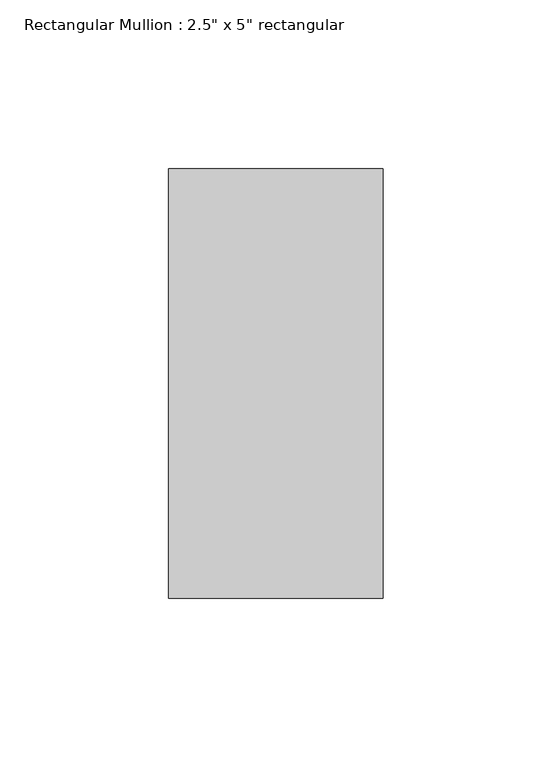
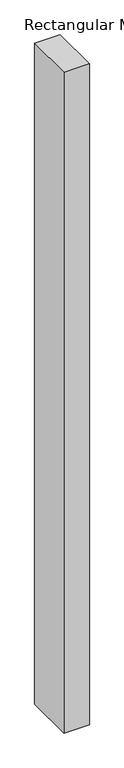
"""IFC4 building model written with IfcOpenShell, lengths in millimetres: member geometry."""

from ifc_helpers import new_model, si_unit, frame, origin, place, context, project, spatial, polyline, outline, extrude, source, transform, mapped, element, save


def member_1bc4b407(model_context):
    return source(origin(), model_context, "Body", "SweptSolid", [
        extrude(outline(polyline([(0.0, 63.5), (0.0, -63.5), (-63.5, -63.5), (-63.5, 63.5), (0.0, 63.5)])), frame((0.0, 0.0, -1750.3622634), z_axis=(0.0, 0.0, 1.0), x_axis=(1.0, 0.0, 0.0)), (0.0, 0.0, 1.0), 1750.3622634),
    ])


if __name__ == "__main__":
    model = new_model("IFC4")
    model_context = context("Model", 3, world=origin())
    ifc_project = project(units=[si_unit("LENGTHUNIT", "METRE", prefix="MILLI")], contexts=[model_context])
    site = spatial("IfcSite", under=ifc_project)
    building = spatial("IfcBuilding", under=site)
    placement = place(None, origin())
    member_shape = member_1bc4b407(model_context)
    element("IfcMember", 1, ObjectType="Rectangular Mullion : 2.5\" x 5\" rectangular", at=placement, inside=building, context=model_context, shape_type="MappedRepresentation", body=[
        mapped(member_shape, transform((0.0, 0.0, 0.0), x_axis=(1.0, 0.0, 0.0), y_axis=(0.0, 1.0, 0.0), z_axis=(0.0, 0.0, 1.0))),
    ])
    save(model, "model.ifc")

# Revit data of these elements
# Type "Rectangular Mullion : 2.5\" x 5\" rectangular"
#   built-in parameter 1007304 = 0.416667 (stored number, unit not read)
#   built-in parameter 1007301 = 0.104167 (stored number, unit not read)
#   built-in parameter 1007300 = 0.104167 (stored number, unit not read)
# Element 1 (IfcMember, "Rectangular Mullion : 2.5\" x 5\" rectangular")
#   Materials on its faces: "Aluminum"
# Materials
#   "Aluminum": class "Metal", colour RGB 247 247 247, transparency 0, Description = "Aluminum 6061", Cost = 0
